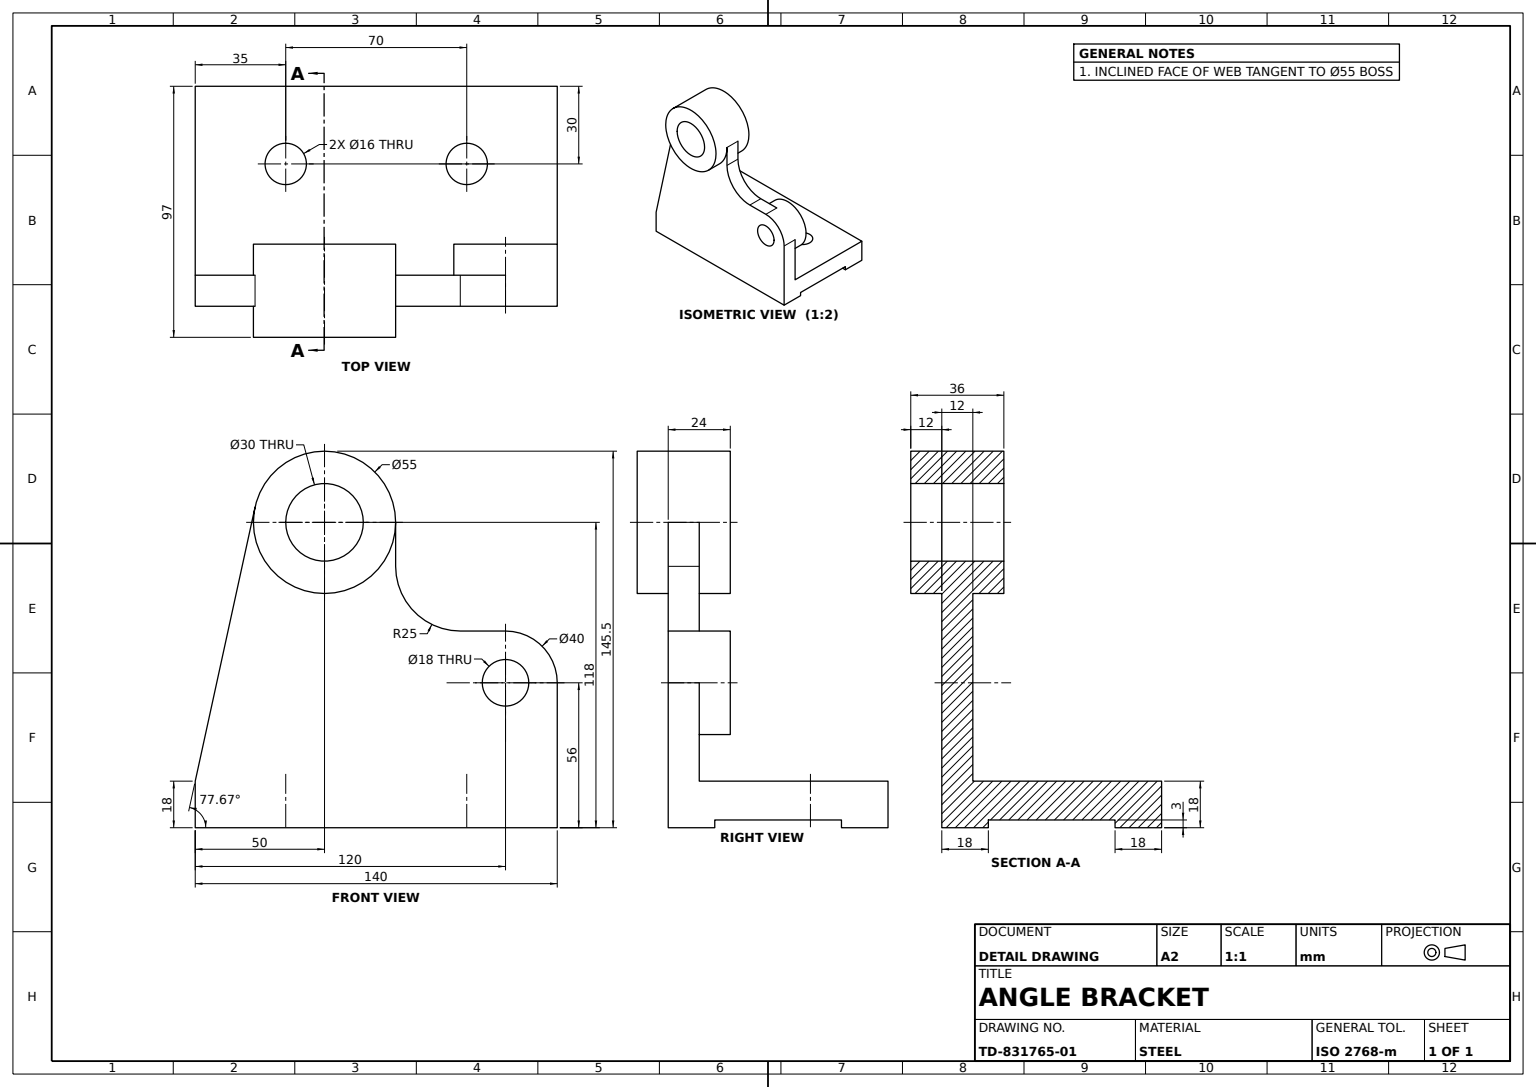
from build123d import *

# Parameters (mm, degrees)
BASE_ANGLE_DEPTH           = 70
PILLAR_WEB_SKETCH_R        = 15
PILLAR_WEB_SKETCH_R_2      = 9
PILLAR_WEB_DEPTH           = 12
BOSS_PROFILES_SKETCH_R     = 9
UPPER_BEARING_BOSS_DEPTH   = 12
LOWER_HUB_BOSS_DEPTH       = 12
LOWER_HUB_BOSS_DEPTH_BACK  = 24
SKETCH5_5_R                = 15
BASE_CUT_REACH             = 157.327
BASE_CUT_SKETCH_R          = 8
BASE_CUT_DIRECTION_2_DEPTH = 156.327074266


with BuildPart() as part:
    # Base Angle Profile Sketch → Base Angle (new, symmetric)
    with BuildSketch(Plane(origin=(0, 0, 0), x_dir=(0, 0, -1), z_dir=(1, 0, 0))):
        Polygon((-24.5, -9), (-24.5, -6), (24.5, -6), (24.5, -9), (42.5, -9), (42.5, 9), (-42.5, 9), (-42.5, -9), align=None)
    extrude(amount=BASE_ANGLE_DEPTH, both=True)

    # Pillar Web Sketch → Pillar Web (add)
    with BuildSketch(Plane(origin=(0, 0, 42.5), x_dir=(-1, 0, 0), z_dir=(0, 0, -1))):
        with BuildLine():
            Line((-70, 47), (-70, 9))
            Line((-70, 9), (70, 9))
            Line((70, 9), (46.866088482, 114.870544241))
            ThreePointArc((46.866088482, 114.870544241), (17.047664759, 136.341062829), (-7.5, 109))
            Line((-7.5, 109), (-7.5, 92))
            ThreePointArc((-7.5, 92), (-14.82233047, 74.32233047), (-32.5, 67))
            Line((-32.5, 67), (-50, 67))
            ThreePointArc((-50, 67), (-64.142135624, 61.142135624), (-70, 47))
        make_face()
        with Locations((20, 109)):
            Circle(PILLAR_WEB_SKETCH_R, mode=Mode.SUBTRACT)
        with Locations((-50, 47)):
            Circle(PILLAR_WEB_SKETCH_R_2, mode=Mode.SUBTRACT)
    extrude(amount=PILLAR_WEB_DEPTH)

    # Boss Profiles Sketch → Upper Bearing Boss (add)
    with BuildSketch(Plane(origin=(0, 0, 30.5), x_dir=(-1, 0, 0), z_dir=(0, 0, -1))):
        with BuildLine():
            ThreePointArc((-70, 47), (-50, 27), (-30, 47))
            ThreePointArc((-30, 47), (-35.857864376, 61.142135624), (-50, 67))
            ThreePointArc((-50, 67), (-64.142135624, 61.142135624), (-70, 47))
        make_face()
        with Locations((-50, 47)):
            Circle(BOSS_PROFILES_SKETCH_R, mode=Mode.SUBTRACT)
    extrude(amount=UPPER_BEARING_BOSS_DEPTH)

    # Sketch5_5 → Lower Hub Boss (add, two sides: drawn at the far end of the back side and taken through both)
    with BuildSketch(Plane(origin=(0, 0, 30.5), x_dir=(-1, 0, 0), z_dir=(0, 0, -1)).offset(-LOWER_HUB_BOSS_DEPTH_BACK)):
        with BuildLine():
            ThreePointArc((-7.5, 109), (20, 81.5), (47.5, 109))
            ThreePointArc((47.5, 109), (47.341062829, 111.952335241), (46.866088482, 114.870544241))
            ThreePointArc((46.866088482, 114.870544241), (17.047664759, 136.341062829), (-7.5, 109))
        make_face()
        with Locations((20, 109)):
            Circle(SKETCH5_5_R, mode=Mode.SUBTRACT)
    extrude(amount=LOWER_HUB_BOSS_DEPTH + LOWER_HUB_BOSS_DEPTH_BACK)

    # Base Cut Sketch → Base Cut (cut, up to next)
    with BuildSketch(Plane(origin=(0, 9, 0), x_dir=(1, 0, 0), z_dir=(0, 1, 0)), mode=Mode.PRIVATE) as base_cut_sk1:
        with Locations(Location((-35, 12.5, 0), (0, 0, 90))):
            Circle(BASE_CUT_SKETCH_R)
    base_cut_tool1 = extrude(base_cut_sk1.sketch, amount=-BASE_CUT_REACH, mode=Mode.PRIVATE) & part.part
    # Base Cut Sketch → Base Cut (cut, up to next)
    with BuildSketch(Plane(origin=(0, 9, 0), x_dir=(1, 0, 0), z_dir=(0, 1, 0)), mode=Mode.PRIVATE) as base_cut_sk2:
        with Locations(Location((35, 12.5, 0), (0, 0, 90))):
            Circle(BASE_CUT_SKETCH_R)
    base_cut_tool2 = extrude(base_cut_sk2.sketch, amount=-BASE_CUT_REACH, mode=Mode.PRIVATE) & part.part
    add(base_cut_tool1.solids().sort_by_distance((-35, 9, -12.5))[0], mode=Mode.SUBTRACT)
    add(base_cut_tool2.solids().sort_by_distance((35, 9, -12.5))[0], mode=Mode.SUBTRACT)

    # Base Cut Sketch → Base Cut direction 2 (cut)
    with BuildSketch(Plane(origin=(0, 9, 0), x_dir=(1, 0, 0), z_dir=(0, 1, 0))):
        with Locations(Location((-35, 12.5, 0), (0, 0, 90))):
            Circle(BASE_CUT_SKETCH_R)
        with Locations(Location((35, 12.5, 0), (0, 0, 90))):
            Circle(BASE_CUT_SKETCH_R)
    extrude(amount=BASE_CUT_DIRECTION_2_DEPTH, mode=Mode.SUBTRACT)


solid = part.part
